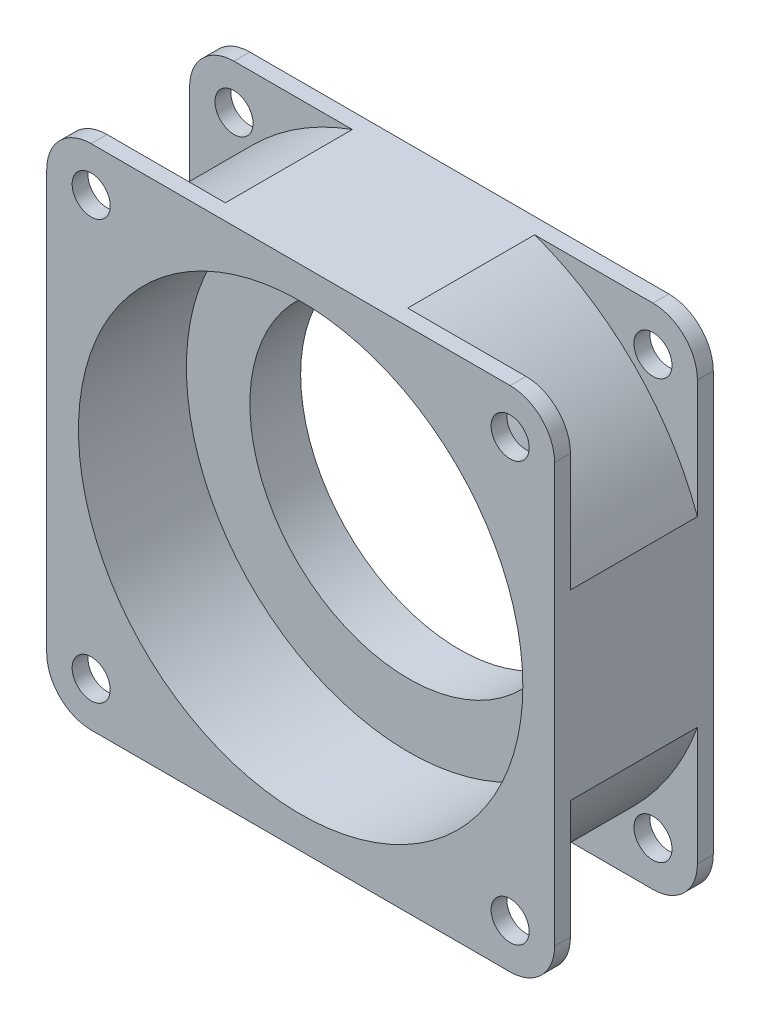
ISO-10303-21;
HEADER;
FILE_DESCRIPTION(('STEP AP214'),'2;1');
FILE_NAME('part.step','',(''),(''),'','','');
FILE_SCHEMA(('AUTOMOTIVE_DESIGN { 1 0 10303 214 1 1 1 1 }'));
ENDSEC;
DATA;
#1=APPLICATION_CONTEXT('core data for automotive mechanical design processes');
#2=APPLICATION_PROTOCOL_DEFINITION('international standard','automotive_design',2000,#1);
#3=PRODUCT_CONTEXT('',#1,'mechanical');
#4=PRODUCT('Part','Part','',(#3));
#5=PRODUCT_RELATED_PRODUCT_CATEGORY('part','',(#4));
#6=PRODUCT_DEFINITION_FORMATION('','',#4);
#7=PRODUCT_DEFINITION_CONTEXT('part definition',#1,'design');
#8=PRODUCT_DEFINITION('design','',#6,#7);
#9=PRODUCT_DEFINITION_SHAPE('','',#8);
#10=(LENGTH_UNIT() NAMED_UNIT(*) SI_UNIT(.MILLI.,.METRE.));
#11=(NAMED_UNIT(*) PLANE_ANGLE_UNIT() SI_UNIT($,.RADIAN.));
#12=(NAMED_UNIT(*) SI_UNIT($,.STERADIAN.) SOLID_ANGLE_UNIT());
#13=UNCERTAINTY_MEASURE_WITH_UNIT(LENGTH_MEASURE(1.E-05),#10,'distance_accuracy_value','');
#14=(GEOMETRIC_REPRESENTATION_CONTEXT(3) GLOBAL_UNCERTAINTY_ASSIGNED_CONTEXT((#13)) GLOBAL_UNIT_ASSIGNED_CONTEXT((#10,
#11,#12)) REPRESENTATION_CONTEXT('',''));
#15=CARTESIAN_POINT('',(0.,0.,0.));
#16=DIRECTION('',(0.,0.,1.));
#17=DIRECTION('',(1.,0.,0.));
#18=AXIS2_PLACEMENT_3D('',#15,#16,#17);
#19=CARTESIAN_POINT('',(0.,0.,-132.5));
#20=DIRECTION('',(0.,0.,1.));
#21=DIRECTION('',(1.,0.,0.));
#22=AXIS2_PLACEMENT_3D('',#19,#20,#21);
#23=CYLINDRICAL_SURFACE('',#22,25.);
#24=CARTESIAN_POINT('',(0.,0.,-25.));
#25=DIRECTION('',(0.,0.,-1.));
#26=DIRECTION('',(-1.,0.,0.));
#27=AXIS2_PLACEMENT_3D('',#24,#25,#26);
#28=CIRCLE('',#27,25.);
#29=CARTESIAN_POINT('',(-25.,0.,-25.));
#30=VERTEX_POINT('',#29);
#31=EDGE_CURVE('E363',#30,#30,#28,.T.);
#32=ORIENTED_EDGE('',*,*,#31,.T.);
#33=EDGE_LOOP('',(#32));
#34=FACE_BOUND('',#33,.T.);
#35=CARTESIAN_POINT('',(0.,0.,-17.));
#36=DIRECTION('',(0.,0.,1.));
#37=DIRECTION('',(1.,0.,0.));
#38=AXIS2_PLACEMENT_3D('',#35,#36,#37);
#39=CIRCLE('',#38,25.);
#40=CARTESIAN_POINT('',(25.,0.,-17.));
#41=VERTEX_POINT('',#40);
#42=EDGE_CURVE('E43',#41,#41,#39,.F.);
#43=ORIENTED_EDGE('',*,*,#42,.F.);
#44=EDGE_LOOP('',(#43));
#45=FACE_BOUND('',#44,.T.);
#46=ADVANCED_FACE('F39',(#34,#45),#23,.F.);
#47=CARTESIAN_POINT('',(33.,33.,-2.5));
#48=DIRECTION('',(0.,0.,-1.));
#49=DIRECTION('',(-1.,0.,0.));
#50=AXIS2_PLACEMENT_3D('',#47,#48,#49);
#51=PLANE('',#50);
#52=CARTESIAN_POINT('',(-33.,33.,-2.5));
#53=DIRECTION('',(0.,0.,-1.));
#54=DIRECTION('',(-1.,0.,0.));
#55=AXIS2_PLACEMENT_3D('',#52,#53,#54);
#56=CIRCLE('',#55,3.);
#57=CARTESIAN_POINT('',(-36.,33.,-2.5));
#58=VERTEX_POINT('',#57);
#59=EDGE_CURVE('E359',#58,#58,#56,.T.);
#60=ORIENTED_EDGE('',*,*,#59,.F.);
#61=EDGE_LOOP('',(#60));
#62=FACE_BOUND('',#61,.T.);
#63=CARTESIAN_POINT('',(0.,0.,-2.5));
#64=DIRECTION('',(0.,0.,-1.));
#65=DIRECTION('',(-1.,0.,0.));
#66=AXIS2_PLACEMENT_3D('',#63,#64,#65);
#67=CIRCLE('',#66,42.5);
#68=CARTESIAN_POINT('',(-40.,14.3614066163451,-2.5));
#69=VERTEX_POINT('',#68);
#70=CARTESIAN_POINT('',(-14.3614066163451,40.,-2.5));
#71=VERTEX_POINT('',#70);
#72=EDGE_CURVE('E229',#69,#71,#67,.T.);
#73=ORIENTED_EDGE('',*,*,#72,.F.);
#74=DIRECTION('',(0.,-1.,0.));
#75=VECTOR('',#74,1.);
#76=CARTESIAN_POINT('',(-40.,-33.,-2.5));
#77=LINE('',#76,#75);
#78=CARTESIAN_POINT('',(-40.,33.,-2.5));
#79=VERTEX_POINT('',#78);
#80=EDGE_CURVE('E287',#79,#69,#77,.T.);
#81=ORIENTED_EDGE('',*,*,#80,.F.);
#82=CARTESIAN_POINT('',(-33.,33.,-2.5));
#83=DIRECTION('',(0.,0.,1.));
#84=DIRECTION('',(-1.,0.,0.));
#85=AXIS2_PLACEMENT_3D('',#82,#83,#84);
#86=CIRCLE('',#85,7.);
#87=CARTESIAN_POINT('',(-32.9999999999999,40.,-2.5));
#88=VERTEX_POINT('',#87);
#89=EDGE_CURVE('E289',#88,#79,#86,.T.);
#90=ORIENTED_EDGE('',*,*,#89,.F.);
#91=DIRECTION('',(-1.,0.,0.));
#92=VECTOR('',#91,1.);
#93=CARTESIAN_POINT('',(-32.9999999999999,40.,-2.5));
#94=LINE('',#93,#92);
#95=EDGE_CURVE('E57',#71,#88,#94,.T.);
#96=ORIENTED_EDGE('',*,*,#95,.F.);
#97=EDGE_LOOP('',(#73,#81,#90,#96));
#98=FACE_BOUND('',#97,.T.);
#99=ADVANCED_FACE('F477',(#62,#98),#51,.T.);
#100=CARTESIAN_POINT('',(-33.,-33.,-2.5));
#101=DIRECTION('',(0.,0.,-1.));
#102=DIRECTION('',(-1.,0.,0.));
#103=AXIS2_PLACEMENT_3D('',#100,#101,#102);
#104=CIRCLE('',#103,3.);
#105=CARTESIAN_POINT('',(-36.,-33.,-2.5));
#106=VERTEX_POINT('',#105);
#107=EDGE_CURVE('E352',#106,#106,#104,.T.);
#108=ORIENTED_EDGE('',*,*,#107,.F.);
#109=EDGE_LOOP('',(#108));
#110=FACE_BOUND('',#109,.T.);
#111=CARTESIAN_POINT('',(0.,0.,-2.5));
#112=DIRECTION('',(0.,0.,-1.));
#113=DIRECTION('',(-1.,0.,0.));
#114=AXIS2_PLACEMENT_3D('',#111,#112,#113);
#115=CIRCLE('',#114,42.5);
#116=CARTESIAN_POINT('',(-14.3614066163451,-40.,-2.5));
#117=VERTEX_POINT('',#116);
#118=CARTESIAN_POINT('',(-40.,-14.3614066163451,-2.5));
#119=VERTEX_POINT('',#118);
#120=EDGE_CURVE('E242',#117,#119,#115,.T.);
#121=ORIENTED_EDGE('',*,*,#120,.F.);
#122=DIRECTION('',(1.,0.,0.));
#123=VECTOR('',#122,1.);
#124=CARTESIAN_POINT('',(-32.9999999999999,-40.,-2.5));
#125=LINE('',#124,#123);
#126=CARTESIAN_POINT('',(-32.9999999999999,-40.,-2.5));
#127=VERTEX_POINT('',#126);
#128=EDGE_CURVE('E300',#127,#117,#125,.T.);
#129=ORIENTED_EDGE('',*,*,#128,.F.);
#130=CARTESIAN_POINT('',(-33.,-33.,-2.5));
#131=DIRECTION('',(0.,0.,1.));
#132=DIRECTION('',(-1.,0.,0.));
#133=AXIS2_PLACEMENT_3D('',#130,#131,#132);
#134=CIRCLE('',#133,7.);
#135=CARTESIAN_POINT('',(-40.,-33.,-2.5));
#136=VERTEX_POINT('',#135);
#137=EDGE_CURVE('E291',#136,#127,#134,.T.);
#138=ORIENTED_EDGE('',*,*,#137,.F.);
#139=EDGE_CURVE('E288',#119,#136,#77,.T.);
#140=ORIENTED_EDGE('',*,*,#139,.F.);
#141=EDGE_LOOP('',(#121,#129,#138,#140));
#142=FACE_BOUND('',#141,.T.);
#143=ADVANCED_FACE('F472',(#110,#142),#51,.T.);
#144=CARTESIAN_POINT('',(33.,-33.,-2.5));
#145=DIRECTION('',(0.,0.,-1.));
#146=DIRECTION('',(-1.,0.,0.));
#147=AXIS2_PLACEMENT_3D('',#144,#145,#146);
#148=CIRCLE('',#147,3.);
#149=CARTESIAN_POINT('',(30.,-33.,-2.5));
#150=VERTEX_POINT('',#149);
#151=EDGE_CURVE('E405',#150,#150,#148,.T.);
#152=ORIENTED_EDGE('',*,*,#151,.F.);
#153=EDGE_LOOP('',(#152));
#154=FACE_BOUND('',#153,.T.);
#155=CARTESIAN_POINT('',(0.,0.,-2.5));
#156=DIRECTION('',(0.,0.,-1.));
#157=DIRECTION('',(-1.,0.,0.));
#158=AXIS2_PLACEMENT_3D('',#155,#156,#157);
#159=CIRCLE('',#158,42.5);
#160=CARTESIAN_POINT('',(40.,-14.3614066163451,-2.5));
#161=VERTEX_POINT('',#160);
#162=CARTESIAN_POINT('',(14.3614066163451,-40.,-2.5));
#163=VERTEX_POINT('',#162);
#164=EDGE_CURVE('E252',#161,#163,#159,.T.);
#165=ORIENTED_EDGE('',*,*,#164,.F.);
#166=DIRECTION('',(0.,1.,0.));
#167=VECTOR('',#166,1.);
#168=CARTESIAN_POINT('',(40.,-33.,-2.5));
#169=LINE('',#168,#167);
#170=CARTESIAN_POINT('',(40.,-33.,-2.5));
#171=VERTEX_POINT('',#170);
#172=EDGE_CURVE('E303',#171,#161,#169,.T.);
#173=ORIENTED_EDGE('',*,*,#172,.F.);
#174=CARTESIAN_POINT('',(33.,-33.,-2.5));
#175=DIRECTION('',(0.,0.,1.));
#176=DIRECTION('',(-1.,0.,0.));
#177=AXIS2_PLACEMENT_3D('',#174,#175,#176);
#178=CIRCLE('',#177,7.);
#179=CARTESIAN_POINT('',(33.,-40.,-2.5));
#180=VERTEX_POINT('',#179);
#181=EDGE_CURVE('E296',#180,#171,#178,.T.);
#182=ORIENTED_EDGE('',*,*,#181,.F.);
#183=EDGE_CURVE('E297',#163,#180,#125,.T.);
#184=ORIENTED_EDGE('',*,*,#183,.F.);
#185=EDGE_LOOP('',(#165,#173,#182,#184));
#186=FACE_BOUND('',#185,.T.);
#187=ADVANCED_FACE('F692',(#154,#186),#51,.T.);
#188=CARTESIAN_POINT('',(33.,33.,-2.5));
#189=DIRECTION('',(0.,0.,1.));
#190=DIRECTION('',(1.,0.,0.));
#191=AXIS2_PLACEMENT_3D('',#188,#189,#190);
#192=CYLINDRICAL_SURFACE('',#191,7.);
#193=CARTESIAN_POINT('',(33.,33.,0.));
#194=DIRECTION('',(0.,0.,1.));
#195=DIRECTION('',(-1.,0.,0.));
#196=AXIS2_PLACEMENT_3D('',#193,#194,#195);
#197=CIRCLE('',#196,7.);
#198=CARTESIAN_POINT('',(40.,33.,0.));
#199=VERTEX_POINT('',#198);
#200=CARTESIAN_POINT('',(33.,40.,0.));
#201=VERTEX_POINT('',#200);
#202=EDGE_CURVE('E276',#199,#201,#197,.T.);
#203=ORIENTED_EDGE('',*,*,#202,.F.);
#204=DIRECTION('',(0.,0.,1.));
#205=VECTOR('',#204,1.);
#206=CARTESIAN_POINT('',(40.,33.,-2.5));
#207=LINE('',#206,#205);
#208=CARTESIAN_POINT('',(40.,33.,-2.5));
#209=VERTEX_POINT('',#208);
#210=EDGE_CURVE('E11',#209,#199,#207,.T.);
#211=ORIENTED_EDGE('',*,*,#210,.F.);
#212=CARTESIAN_POINT('',(33.,33.,-2.5));
#213=DIRECTION('',(0.,0.,1.));
#214=DIRECTION('',(-1.,0.,0.));
#215=AXIS2_PLACEMENT_3D('',#212,#213,#214);
#216=CIRCLE('',#215,7.);
#217=CARTESIAN_POINT('',(33.,40.,-2.5));
#218=VERTEX_POINT('',#217);
#219=EDGE_CURVE('E278',#209,#218,#216,.T.);
#220=ORIENTED_EDGE('',*,*,#219,.T.);
#221=DIRECTION('',(0.,0.,1.));
#222=VECTOR('',#221,1.);
#223=CARTESIAN_POINT('',(33.,40.,-2.5));
#224=LINE('',#223,#222);
#225=EDGE_CURVE('E307',#218,#201,#224,.T.);
#226=ORIENTED_EDGE('',*,*,#225,.T.);
#227=EDGE_LOOP('',(#203,#211,#220,#226));
#228=FACE_BOUND('',#227,.T.);
#229=ADVANCED_FACE('F41',(#228),#192,.T.);
#230=CARTESIAN_POINT('',(40.,-33.,-2.5));
#231=DIRECTION('',(1.,0.,0.));
#232=DIRECTION('',(0.,0.,-1.));
#233=AXIS2_PLACEMENT_3D('',#230,#231,#232);
#234=PLANE('',#233);
#235=DIRECTION('',(0.,1.,0.));
#236=VECTOR('',#235,1.);
#237=CARTESIAN_POINT('',(40.,-33.,0.));
#238=LINE('',#237,#236);
#239=CARTESIAN_POINT('',(40.,-33.,0.));
#240=VERTEX_POINT('',#239);
#241=EDGE_CURVE('E283',#240,#199,#238,.T.);
#242=ORIENTED_EDGE('',*,*,#241,.F.);
#243=DIRECTION('',(0.,0.,1.));
#244=VECTOR('',#243,1.);
#245=CARTESIAN_POINT('',(40.,-33.,-2.5));
#246=LINE('',#245,#244);
#247=EDGE_CURVE('E48',#171,#240,#246,.T.);
#248=ORIENTED_EDGE('',*,*,#247,.F.);
#249=ORIENTED_EDGE('',*,*,#172,.T.);
#250=DIRECTION('',(0.,0.,1.));
#251=VECTOR('',#250,1.);
#252=CARTESIAN_POINT('',(40.,-14.3614066163451,-22.5));
#253=LINE('',#252,#251);
#254=CARTESIAN_POINT('',(40.,-14.3614066163451,-22.5));
#255=VERTEX_POINT('',#254);
#256=EDGE_CURVE('E268',#255,#161,#253,.T.);
#257=ORIENTED_EDGE('',*,*,#256,.F.);
#258=DIRECTION('',(0.,-1.,0.));
#259=VECTOR('',#258,1.);
#260=CARTESIAN_POINT('',(40.,-33.,-22.5));
#261=LINE('',#260,#259);
#262=CARTESIAN_POINT('',(40.,-33.,-22.5));
#263=VERTEX_POINT('',#262);
#264=EDGE_CURVE('E432',#255,#263,#261,.T.);
#265=ORIENTED_EDGE('',*,*,#264,.T.);
#266=DIRECTION('',(0.,0.,1.));
#267=VECTOR('',#266,1.);
#268=CARTESIAN_POINT('',(40.,-33.,-25.));
#269=LINE('',#268,#267);
#270=CARTESIAN_POINT('',(40.,-33.,-25.));
#271=VERTEX_POINT('',#270);
#272=EDGE_CURVE('E412',#271,#263,#269,.T.);
#273=ORIENTED_EDGE('',*,*,#272,.F.);
#274=DIRECTION('',(0.,-1.,0.));
#275=VECTOR('',#274,1.);
#276=CARTESIAN_POINT('',(40.,-33.,-25.));
#277=LINE('',#276,#275);
#278=CARTESIAN_POINT('',(40.,32.9999999999999,-25.));
#279=VERTEX_POINT('',#278);
#280=EDGE_CURVE('E219',#279,#271,#277,.T.);
#281=ORIENTED_EDGE('',*,*,#280,.F.);
#282=DIRECTION('',(0.,0.,1.));
#283=VECTOR('',#282,1.);
#284=CARTESIAN_POINT('',(40.,32.9999999999999,-25.));
#285=LINE('',#284,#283);
#286=CARTESIAN_POINT('',(40.,32.9999999999999,-22.5));
#287=VERTEX_POINT('',#286);
#288=EDGE_CURVE('E437',#279,#287,#285,.T.);
#289=ORIENTED_EDGE('',*,*,#288,.T.);
#290=CARTESIAN_POINT('',(40.,14.3614066163451,-22.5));
#291=VERTEX_POINT('',#290);
#292=EDGE_CURVE('E221',#287,#291,#261,.T.);
#293=ORIENTED_EDGE('',*,*,#292,.T.);
#294=DIRECTION('',(0.,0.,1.));
#295=VECTOR('',#294,1.);
#296=CARTESIAN_POINT('',(40.,14.3614066163451,-22.5));
#297=LINE('',#296,#295);
#298=CARTESIAN_POINT('',(40.,14.3614066163451,-2.5));
#299=VERTEX_POINT('',#298);
#300=EDGE_CURVE('E271',#291,#299,#297,.T.);
#301=ORIENTED_EDGE('',*,*,#300,.T.);
#302=EDGE_CURVE('E305',#299,#209,#169,.T.);
#303=ORIENTED_EDGE('',*,*,#302,.T.);
#304=ORIENTED_EDGE('',*,*,#210,.T.);
#305=EDGE_LOOP('',(#242,#248,#249,#257,#265,#273,#281,#289,#293,#301,#303,#304));
#306=FACE_BOUND('',#305,.T.);
#307=ADVANCED_FACE('F639',(#306),#234,.T.);
#308=CARTESIAN_POINT('',(33.,-33.,-2.5));
#309=DIRECTION('',(0.,0.,1.));
#310=DIRECTION('',(1.,0.,0.));
#311=AXIS2_PLACEMENT_3D('',#308,#309,#310);
#312=CYLINDRICAL_SURFACE('',#311,7.);
#313=CARTESIAN_POINT('',(33.,-33.,0.));
#314=DIRECTION('',(0.,0.,1.));
#315=DIRECTION('',(-1.,0.,0.));
#316=AXIS2_PLACEMENT_3D('',#313,#314,#315);
#317=CIRCLE('',#316,7.);
#318=CARTESIAN_POINT('',(33.,-40.,0.));
#319=VERTEX_POINT('',#318);
#320=EDGE_CURVE('E324',#319,#240,#317,.T.);
#321=ORIENTED_EDGE('',*,*,#320,.F.);
#322=DIRECTION('',(0.,0.,1.));
#323=VECTOR('',#322,1.);
#324=CARTESIAN_POINT('',(33.,-40.,-2.5));
#325=LINE('',#324,#323);
#326=EDGE_CURVE('E332',#180,#319,#325,.T.);
#327=ORIENTED_EDGE('',*,*,#326,.F.);
#328=ORIENTED_EDGE('',*,*,#181,.T.);
#329=ORIENTED_EDGE('',*,*,#247,.T.);
#330=EDGE_LOOP('',(#321,#327,#328,#329));
#331=FACE_BOUND('',#330,.T.);
#332=ADVANCED_FACE('F631',(#331),#312,.T.);
#333=CARTESIAN_POINT('',(-32.9999999999999,-40.,-2.5));
#334=DIRECTION('',(0.,-1.,0.));
#335=DIRECTION('',(0.,0.,-1.));
#336=AXIS2_PLACEMENT_3D('',#333,#334,#335);
#337=PLANE('',#336);
#338=DIRECTION('',(1.,0.,0.));
#339=VECTOR('',#338,1.);
#340=CARTESIAN_POINT('',(-32.9999999999999,-40.,0.));
#341=LINE('',#340,#339);
#342=CARTESIAN_POINT('',(-32.9999999999999,-40.,0.));
#343=VERTEX_POINT('',#342);
#344=EDGE_CURVE('E325',#343,#319,#341,.T.);
#345=ORIENTED_EDGE('',*,*,#344,.F.);
#346=DIRECTION('',(0.,0.,1.));
#347=VECTOR('',#346,1.);
#348=CARTESIAN_POINT('',(-32.9999999999999,-40.,-2.5));
#349=LINE('',#348,#347);
#350=EDGE_CURVE('E334',#127,#343,#349,.T.);
#351=ORIENTED_EDGE('',*,*,#350,.F.);
#352=ORIENTED_EDGE('',*,*,#128,.T.);
#353=DIRECTION('',(0.,0.,1.));
#354=VECTOR('',#353,1.);
#355=CARTESIAN_POINT('',(-14.3614066163451,-40.,-22.5));
#356=LINE('',#355,#354);
#357=CARTESIAN_POINT('',(-14.3614066163451,-40.,-22.5));
#358=VERTEX_POINT('',#357);
#359=EDGE_CURVE('E265',#358,#117,#356,.T.);
#360=ORIENTED_EDGE('',*,*,#359,.F.);
#361=DIRECTION('',(-1.,0.,0.));
#362=VECTOR('',#361,1.);
#363=CARTESIAN_POINT('',(-33.,-40.,-22.5));
#364=LINE('',#363,#362);
#365=CARTESIAN_POINT('',(-33.,-40.,-22.5));
#366=VERTEX_POINT('',#365);
#367=EDGE_CURVE('E417',#358,#366,#364,.T.);
#368=ORIENTED_EDGE('',*,*,#367,.T.);
#369=DIRECTION('',(0.,0.,1.));
#370=VECTOR('',#369,1.);
#371=CARTESIAN_POINT('',(-33.,-40.,-25.));
#372=LINE('',#371,#370);
#373=CARTESIAN_POINT('',(-33.,-40.,-25.));
#374=VERTEX_POINT('',#373);
#375=EDGE_CURVE('E211',#374,#366,#372,.T.);
#376=ORIENTED_EDGE('',*,*,#375,.F.);
#377=DIRECTION('',(-1.,0.,0.));
#378=VECTOR('',#377,1.);
#379=CARTESIAN_POINT('',(-33.,-40.,-25.));
#380=LINE('',#379,#378);
#381=CARTESIAN_POINT('',(32.9999999999999,-40.,-25.));
#382=VERTEX_POINT('',#381);
#383=EDGE_CURVE('E205',#382,#374,#380,.T.);
#384=ORIENTED_EDGE('',*,*,#383,.F.);
#385=DIRECTION('',(0.,0.,1.));
#386=VECTOR('',#385,1.);
#387=CARTESIAN_POINT('',(32.9999999999999,-40.,-25.));
#388=LINE('',#387,#386);
#389=CARTESIAN_POINT('',(32.9999999999999,-40.,-22.5));
#390=VERTEX_POINT('',#389);
#391=EDGE_CURVE('E208',#382,#390,#388,.T.);
#392=ORIENTED_EDGE('',*,*,#391,.T.);
#393=CARTESIAN_POINT('',(14.3614066163451,-40.,-22.5));
#394=VERTEX_POINT('',#393);
#395=EDGE_CURVE('E416',#390,#394,#364,.T.);
#396=ORIENTED_EDGE('',*,*,#395,.T.);
#397=DIRECTION('',(0.,0.,1.));
#398=VECTOR('',#397,1.);
#399=CARTESIAN_POINT('',(14.3614066163451,-40.,-22.5));
#400=LINE('',#399,#398);
#401=EDGE_CURVE('E264',#394,#163,#400,.T.);
#402=ORIENTED_EDGE('',*,*,#401,.T.);
#403=ORIENTED_EDGE('',*,*,#183,.T.);
#404=ORIENTED_EDGE('',*,*,#326,.T.);
#405=EDGE_LOOP('',(#345,#351,#352,#360,#368,#376,#384,#392,#396,#402,#403,#404));
#406=FACE_BOUND('',#405,.T.);
#407=ADVANCED_FACE('F202',(#406),#337,.T.);
#408=CARTESIAN_POINT('',(-33.,-33.,-2.5));
#409=DIRECTION('',(0.,0.,1.));
#410=DIRECTION('',(1.,0.,0.));
#411=AXIS2_PLACEMENT_3D('',#408,#409,#410);
#412=CYLINDRICAL_SURFACE('',#411,7.);
#413=CARTESIAN_POINT('',(-33.,-33.,0.));
#414=DIRECTION('',(0.,0.,1.));
#415=DIRECTION('',(-1.,0.,0.));
#416=AXIS2_PLACEMENT_3D('',#413,#414,#415);
#417=CIRCLE('',#416,7.);
#418=CARTESIAN_POINT('',(-40.,-33.,0.));
#419=VERTEX_POINT('',#418);
#420=EDGE_CURVE('E317',#419,#343,#417,.T.);
#421=ORIENTED_EDGE('',*,*,#420,.F.);
#422=DIRECTION('',(0.,0.,1.));
#423=VECTOR('',#422,1.);
#424=CARTESIAN_POINT('',(-40.,-33.,-2.5));
#425=LINE('',#424,#423);
#426=EDGE_CURVE('E333',#136,#419,#425,.T.);
#427=ORIENTED_EDGE('',*,*,#426,.F.);
#428=ORIENTED_EDGE('',*,*,#137,.T.);
#429=ORIENTED_EDGE('',*,*,#350,.T.);
#430=EDGE_LOOP('',(#421,#427,#428,#429));
#431=FACE_BOUND('',#430,.T.);
#432=ADVANCED_FACE('F467',(#431),#412,.T.);
#433=CARTESIAN_POINT('',(-40.,-33.,-2.5));
#434=DIRECTION('',(-1.,0.,0.));
#435=DIRECTION('',(0.,0.,1.));
#436=AXIS2_PLACEMENT_3D('',#433,#434,#435);
#437=PLANE('',#436);
#438=DIRECTION('',(0.,-1.,0.));
#439=VECTOR('',#438,1.);
#440=CARTESIAN_POINT('',(-40.,-33.,0.));
#441=LINE('',#440,#439);
#442=CARTESIAN_POINT('',(-40.,33.,0.));
#443=VERTEX_POINT('',#442);
#444=EDGE_CURVE('E316',#443,#419,#441,.T.);
#445=ORIENTED_EDGE('',*,*,#444,.F.);
#446=DIRECTION('',(0.,0.,1.));
#447=VECTOR('',#446,1.);
#448=CARTESIAN_POINT('',(-40.,33.,-2.5));
#449=LINE('',#448,#447);
#450=EDGE_CURVE('E340',#79,#443,#449,.T.);
#451=ORIENTED_EDGE('',*,*,#450,.F.);
#452=ORIENTED_EDGE('',*,*,#80,.T.);
#453=DIRECTION('',(0.,0.,1.));
#454=VECTOR('',#453,1.);
#455=CARTESIAN_POINT('',(-40.,14.3614066163451,-22.5));
#456=LINE('',#455,#454);
#457=CARTESIAN_POINT('',(-40.,14.3614066163451,-22.5));
#458=VERTEX_POINT('',#457);
#459=EDGE_CURVE('E248',#458,#69,#456,.T.);
#460=ORIENTED_EDGE('',*,*,#459,.F.);
#461=DIRECTION('',(0.,1.,0.));
#462=VECTOR('',#461,1.);
#463=CARTESIAN_POINT('',(-40.,-33.,-22.5));
#464=LINE('',#463,#462);
#465=CARTESIAN_POINT('',(-40.,33.,-22.5));
#466=VERTEX_POINT('',#465);
#467=EDGE_CURVE('E425',#458,#466,#464,.T.);
#468=ORIENTED_EDGE('',*,*,#467,.T.);
#469=DIRECTION('',(0.,0.,1.));
#470=VECTOR('',#469,1.);
#471=CARTESIAN_POINT('',(-40.,33.,-25.));
#472=LINE('',#471,#470);
#473=CARTESIAN_POINT('',(-40.,33.,-25.));
#474=VERTEX_POINT('',#473);
#475=EDGE_CURVE('E450',#474,#466,#472,.T.);
#476=ORIENTED_EDGE('',*,*,#475,.F.);
#477=DIRECTION('',(0.,1.,0.));
#478=VECTOR('',#477,1.);
#479=CARTESIAN_POINT('',(-40.,-33.,-25.));
#480=LINE('',#479,#478);
#481=CARTESIAN_POINT('',(-40.,-33.,-25.));
#482=VERTEX_POINT('',#481);
#483=EDGE_CURVE('E407',#482,#474,#480,.T.);
#484=ORIENTED_EDGE('',*,*,#483,.F.);
#485=DIRECTION('',(0.,0.,1.));
#486=VECTOR('',#485,1.);
#487=CARTESIAN_POINT('',(-40.,-33.,-25.));
#488=LINE('',#487,#486);
#489=CARTESIAN_POINT('',(-40.,-33.,-22.5));
#490=VERTEX_POINT('',#489);
#491=EDGE_CURVE('E235',#482,#490,#488,.T.);
#492=ORIENTED_EDGE('',*,*,#491,.T.);
#493=CARTESIAN_POINT('',(-40.,-14.3614066163451,-22.5));
#494=VERTEX_POINT('',#493);
#495=EDGE_CURVE('E421',#490,#494,#464,.T.);
#496=ORIENTED_EDGE('',*,*,#495,.T.);
#497=DIRECTION('',(0.,0.,1.));
#498=VECTOR('',#497,1.);
#499=CARTESIAN_POINT('',(-40.,-14.3614066163451,-22.5));
#500=LINE('',#499,#498);
#501=EDGE_CURVE('E259',#494,#119,#500,.T.);
#502=ORIENTED_EDGE('',*,*,#501,.T.);
#503=ORIENTED_EDGE('',*,*,#139,.T.);
#504=ORIENTED_EDGE('',*,*,#426,.T.);
#505=EDGE_LOOP('',(#445,#451,#452,#460,#468,#476,#484,#492,#496,#502,#503,#504));
#506=FACE_BOUND('',#505,.T.);
#507=ADVANCED_FACE('F452',(#506),#437,.T.);
#508=CARTESIAN_POINT('',(-33.,33.,-2.5));
#509=DIRECTION('',(0.,0.,1.));
#510=DIRECTION('',(1.,0.,0.));
#511=AXIS2_PLACEMENT_3D('',#508,#509,#510);
#512=CYLINDRICAL_SURFACE('',#511,7.);
#513=CARTESIAN_POINT('',(-33.,33.,0.));
#514=DIRECTION('',(0.,0.,1.));
#515=DIRECTION('',(-1.,0.,0.));
#516=AXIS2_PLACEMENT_3D('',#513,#514,#515);
#517=CIRCLE('',#516,7.);
#518=CARTESIAN_POINT('',(-32.9999999999999,40.,0.));
#519=VERTEX_POINT('',#518);
#520=EDGE_CURVE('E311',#519,#443,#517,.T.);
#521=ORIENTED_EDGE('',*,*,#520,.F.);
#522=DIRECTION('',(0.,0.,1.));
#523=VECTOR('',#522,1.);
#524=CARTESIAN_POINT('',(-32.9999999999999,40.,-2.5));
#525=LINE('',#524,#523);
#526=EDGE_CURVE('E339',#88,#519,#525,.T.);
#527=ORIENTED_EDGE('',*,*,#526,.F.);
#528=ORIENTED_EDGE('',*,*,#89,.T.);
#529=ORIENTED_EDGE('',*,*,#450,.T.);
#530=EDGE_LOOP('',(#521,#527,#528,#529));
#531=FACE_BOUND('',#530,.T.);
#532=ADVANCED_FACE('F485',(#531),#512,.T.);
#533=CARTESIAN_POINT('',(-32.9999999999999,40.,-2.5));
#534=DIRECTION('',(0.,1.,0.));
#535=DIRECTION('',(0.,0.,1.));
#536=AXIS2_PLACEMENT_3D('',#533,#534,#535);
#537=PLANE('',#536);
#538=DIRECTION('',(-1.,0.,0.));
#539=VECTOR('',#538,1.);
#540=CARTESIAN_POINT('',(-32.9999999999999,40.,0.));
#541=LINE('',#540,#539);
#542=EDGE_CURVE('E309',#201,#519,#541,.T.);
#543=ORIENTED_EDGE('',*,*,#542,.F.);
#544=ORIENTED_EDGE('',*,*,#225,.F.);
#545=CARTESIAN_POINT('',(14.3614066163451,40.,-2.5));
#546=VERTEX_POINT('',#545);
#547=EDGE_CURVE('E284',#218,#546,#94,.T.);
#548=ORIENTED_EDGE('',*,*,#547,.T.);
#549=DIRECTION('',(0.,0.,1.));
#550=VECTOR('',#549,1.);
#551=CARTESIAN_POINT('',(14.3614066163451,40.,-22.5));
#552=LINE('',#551,#550);
#553=CARTESIAN_POINT('',(14.3614066163451,40.,-22.5));
#554=VERTEX_POINT('',#553);
#555=EDGE_CURVE('E273',#554,#546,#552,.T.);
#556=ORIENTED_EDGE('',*,*,#555,.F.);
#557=DIRECTION('',(1.,0.,0.));
#558=VECTOR('',#557,1.);
#559=CARTESIAN_POINT('',(-33.,40.,-22.5));
#560=LINE('',#559,#558);
#561=CARTESIAN_POINT('',(32.9999999999999,40.,-22.5));
#562=VERTEX_POINT('',#561);
#563=EDGE_CURVE('E428',#554,#562,#560,.T.);
#564=ORIENTED_EDGE('',*,*,#563,.T.);
#565=DIRECTION('',(0.,0.,1.));
#566=VECTOR('',#565,1.);
#567=CARTESIAN_POINT('',(32.9999999999999,40.,-25.));
#568=LINE('',#567,#566);
#569=CARTESIAN_POINT('',(32.9999999999999,40.,-25.));
#570=VERTEX_POINT('',#569);
#571=EDGE_CURVE('E442',#570,#562,#568,.T.);
#572=ORIENTED_EDGE('',*,*,#571,.F.);
#573=DIRECTION('',(1.,0.,0.));
#574=VECTOR('',#573,1.);
#575=CARTESIAN_POINT('',(-33.,40.,-25.));
#576=LINE('',#575,#574);
#577=CARTESIAN_POINT('',(-33.,40.,-25.));
#578=VERTEX_POINT('',#577);
#579=EDGE_CURVE('E406',#578,#570,#576,.T.);
#580=ORIENTED_EDGE('',*,*,#579,.F.);
#581=DIRECTION('',(0.,0.,1.));
#582=VECTOR('',#581,1.);
#583=CARTESIAN_POINT('',(-33.,40.,-25.));
#584=LINE('',#583,#582);
#585=CARTESIAN_POINT('',(-33.,40.,-22.5));
#586=VERTEX_POINT('',#585);
#587=EDGE_CURVE('E441',#578,#586,#584,.T.);
#588=ORIENTED_EDGE('',*,*,#587,.T.);
#589=CARTESIAN_POINT('',(-14.3614066163451,40.,-22.5));
#590=VERTEX_POINT('',#589);
#591=EDGE_CURVE('E427',#586,#590,#560,.T.);
#592=ORIENTED_EDGE('',*,*,#591,.T.);
#593=DIRECTION('',(0.,0.,1.));
#594=VECTOR('',#593,1.);
#595=CARTESIAN_POINT('',(-14.3614066163451,40.,-22.5));
#596=LINE('',#595,#594);
#597=EDGE_CURVE('E280',#590,#71,#596,.T.);
#598=ORIENTED_EDGE('',*,*,#597,.T.);
#599=ORIENTED_EDGE('',*,*,#95,.T.);
#600=ORIENTED_EDGE('',*,*,#526,.T.);
#601=EDGE_LOOP('',(#543,#544,#548,#556,#564,#572,#580,#588,#592,#598,#599,#600));
#602=FACE_BOUND('',#601,.T.);
#603=ADVANCED_FACE('F484',(#602),#537,.T.);
#604=CARTESIAN_POINT('',(33.,33.,-2.5));
#605=DIRECTION('',(0.,0.,-1.));
#606=DIRECTION('',(-1.,0.,0.));
#607=AXIS2_PLACEMENT_3D('',#604,#605,#606);
#608=CIRCLE('',#607,3.);
#609=CARTESIAN_POINT('',(30.,33.,-2.5));
#610=VERTEX_POINT('',#609);
#611=EDGE_CURVE('E357',#610,#610,#608,.T.);
#612=ORIENTED_EDGE('',*,*,#611,.F.);
#613=EDGE_LOOP('',(#612));
#614=FACE_BOUND('',#613,.T.);
#615=CARTESIAN_POINT('',(0.,0.,-2.5));
#616=DIRECTION('',(0.,0.,-1.));
#617=DIRECTION('',(-1.,0.,0.));
#618=AXIS2_PLACEMENT_3D('',#615,#616,#617);
#619=CIRCLE('',#618,42.5);
#620=EDGE_CURVE('E64',#546,#299,#619,.T.);
#621=ORIENTED_EDGE('',*,*,#620,.F.);
#622=ORIENTED_EDGE('',*,*,#547,.F.);
#623=ORIENTED_EDGE('',*,*,#219,.F.);
#624=ORIENTED_EDGE('',*,*,#302,.F.);
#625=EDGE_LOOP('',(#621,#622,#623,#624));
#626=FACE_BOUND('',#625,.T.);
#627=ADVANCED_FACE('F522',(#614,#626),#51,.T.);
#628=CARTESIAN_POINT('',(33.,33.,0.));
#629=DIRECTION('',(0.,0.,-1.));
#630=DIRECTION('',(-1.,0.,0.));
#631=AXIS2_PLACEMENT_3D('',#628,#629,#630);
#632=PLANE('',#631);
#633=CARTESIAN_POINT('',(0.,0.,0.));
#634=DIRECTION('',(0.,0.,1.));
#635=DIRECTION('',(1.,0.,0.));
#636=AXIS2_PLACEMENT_3D('',#633,#634,#635);
#637=CIRCLE('',#636,35.);
#638=CARTESIAN_POINT('',(35.,0.,0.));
#639=VERTEX_POINT('',#638);
#640=EDGE_CURVE('E372',#639,#639,#637,.T.);
#641=ORIENTED_EDGE('',*,*,#640,.F.);
#642=EDGE_LOOP('',(#641));
#643=FACE_BOUND('',#642,.T.);
#644=CARTESIAN_POINT('',(-33.,-33.,0.));
#645=DIRECTION('',(0.,0.,1.));
#646=DIRECTION('',(1.,0.,0.));
#647=AXIS2_PLACEMENT_3D('',#644,#645,#646);
#648=CIRCLE('',#647,3.);
#649=CARTESIAN_POINT('',(-30.,-33.,0.));
#650=VERTEX_POINT('',#649);
#651=EDGE_CURVE('E361',#650,#650,#648,.T.);
#652=ORIENTED_EDGE('',*,*,#651,.F.);
#653=EDGE_LOOP('',(#652));
#654=FACE_BOUND('',#653,.T.);
#655=CARTESIAN_POINT('',(33.,-33.,0.));
#656=DIRECTION('',(0.,0.,1.));
#657=DIRECTION('',(1.,0.,0.));
#658=AXIS2_PLACEMENT_3D('',#655,#656,#657);
#659=CIRCLE('',#658,3.);
#660=CARTESIAN_POINT('',(36.,-33.,0.));
#661=VERTEX_POINT('',#660);
#662=EDGE_CURVE('E370',#661,#661,#659,.T.);
#663=ORIENTED_EDGE('',*,*,#662,.F.);
#664=EDGE_LOOP('',(#663));
#665=FACE_BOUND('',#664,.T.);
#666=CARTESIAN_POINT('',(33.,33.,0.));
#667=DIRECTION('',(0.,0.,1.));
#668=DIRECTION('',(1.,0.,0.));
#669=AXIS2_PLACEMENT_3D('',#666,#667,#668);
#670=CIRCLE('',#669,3.);
#671=CARTESIAN_POINT('',(36.,33.,0.));
#672=VERTEX_POINT('',#671);
#673=EDGE_CURVE('E381',#672,#672,#670,.T.);
#674=ORIENTED_EDGE('',*,*,#673,.F.);
#675=EDGE_LOOP('',(#674));
#676=FACE_BOUND('',#675,.T.);
#677=CARTESIAN_POINT('',(-33.,33.,0.));
#678=DIRECTION('',(0.,0.,1.));
#679=DIRECTION('',(1.,0.,0.));
#680=AXIS2_PLACEMENT_3D('',#677,#678,#679);
#681=CIRCLE('',#680,3.);
#682=CARTESIAN_POINT('',(-30.,33.,0.));
#683=VERTEX_POINT('',#682);
#684=EDGE_CURVE('E347',#683,#683,#681,.T.);
#685=ORIENTED_EDGE('',*,*,#684,.F.);
#686=EDGE_LOOP('',(#685));
#687=FACE_BOUND('',#686,.T.);
#688=ORIENTED_EDGE('',*,*,#202,.T.);
#689=ORIENTED_EDGE('',*,*,#542,.T.);
#690=ORIENTED_EDGE('',*,*,#520,.T.);
#691=ORIENTED_EDGE('',*,*,#444,.T.);
#692=ORIENTED_EDGE('',*,*,#420,.T.);
#693=ORIENTED_EDGE('',*,*,#344,.T.);
#694=ORIENTED_EDGE('',*,*,#320,.T.);
#695=ORIENTED_EDGE('',*,*,#241,.T.);
#696=EDGE_LOOP('',(#688,#689,#690,#691,#692,#693,#694,#695));
#697=FACE_BOUND('',#696,.T.);
#698=ADVANCED_FACE('F478',(#643,#654,#665,#676,#687,#697),#632,.F.);
#699=CARTESIAN_POINT('',(0.,0.,-22.5));
#700=DIRECTION('',(0.,0.,1.));
#701=DIRECTION('',(1.,0.,0.));
#702=AXIS2_PLACEMENT_3D('',#699,#700,#701);
#703=CYLINDRICAL_SURFACE('',#702,42.5);
#704=ORIENTED_EDGE('',*,*,#72,.T.);
#705=ORIENTED_EDGE('',*,*,#597,.F.);
#706=CARTESIAN_POINT('',(0.,0.,-22.5));
#707=DIRECTION('',(0.,0.,-1.));
#708=DIRECTION('',(-1.,0.,0.));
#709=AXIS2_PLACEMENT_3D('',#706,#707,#708);
#710=CIRCLE('',#709,42.5);
#711=EDGE_CURVE('E240',#458,#590,#710,.T.);
#712=ORIENTED_EDGE('',*,*,#711,.F.);
#713=ORIENTED_EDGE('',*,*,#459,.T.);
#714=EDGE_LOOP('',(#704,#705,#712,#713));
#715=FACE_BOUND('',#714,.T.);
#716=ADVANCED_FACE('F487',(#715),#703,.T.);
#717=CARTESIAN_POINT('',(0.,0.,-22.5));
#718=DIRECTION('',(0.,0.,1.));
#719=DIRECTION('',(1.,0.,0.));
#720=AXIS2_PLACEMENT_3D('',#717,#718,#719);
#721=CYLINDRICAL_SURFACE('',#720,42.5);
#722=ORIENTED_EDGE('',*,*,#620,.T.);
#723=ORIENTED_EDGE('',*,*,#300,.F.);
#724=CARTESIAN_POINT('',(0.,0.,-22.5));
#725=DIRECTION('',(0.,0.,-1.));
#726=DIRECTION('',(-1.,0.,0.));
#727=AXIS2_PLACEMENT_3D('',#724,#725,#726);
#728=CIRCLE('',#727,42.5);
#729=EDGE_CURVE('E238',#554,#291,#728,.T.);
#730=ORIENTED_EDGE('',*,*,#729,.F.);
#731=ORIENTED_EDGE('',*,*,#555,.T.);
#732=EDGE_LOOP('',(#722,#723,#730,#731));
#733=FACE_BOUND('',#732,.T.);
#734=ADVANCED_FACE('F664',(#733),#721,.T.);
#735=CARTESIAN_POINT('',(0.,0.,-22.5));
#736=DIRECTION('',(0.,0.,1.));
#737=DIRECTION('',(1.,0.,0.));
#738=AXIS2_PLACEMENT_3D('',#735,#736,#737);
#739=CYLINDRICAL_SURFACE('',#738,42.5);
#740=ORIENTED_EDGE('',*,*,#164,.T.);
#741=ORIENTED_EDGE('',*,*,#401,.F.);
#742=CARTESIAN_POINT('',(0.,0.,-22.5));
#743=DIRECTION('',(0.,0.,-1.));
#744=DIRECTION('',(-1.,0.,0.));
#745=AXIS2_PLACEMENT_3D('',#742,#743,#744);
#746=CIRCLE('',#745,42.5);
#747=EDGE_CURVE('E244',#255,#394,#746,.T.);
#748=ORIENTED_EDGE('',*,*,#747,.F.);
#749=ORIENTED_EDGE('',*,*,#256,.T.);
#750=EDGE_LOOP('',(#740,#741,#748,#749));
#751=FACE_BOUND('',#750,.T.);
#752=ADVANCED_FACE('F508',(#751),#739,.T.);
#753=CARTESIAN_POINT('',(0.,0.,-22.5));
#754=DIRECTION('',(0.,0.,1.));
#755=DIRECTION('',(1.,0.,0.));
#756=AXIS2_PLACEMENT_3D('',#753,#754,#755);
#757=CYLINDRICAL_SURFACE('',#756,42.5);
#758=ORIENTED_EDGE('',*,*,#120,.T.);
#759=ORIENTED_EDGE('',*,*,#501,.F.);
#760=CARTESIAN_POINT('',(0.,0.,-22.5));
#761=DIRECTION('',(0.,0.,-1.));
#762=DIRECTION('',(-1.,0.,0.));
#763=AXIS2_PLACEMENT_3D('',#760,#761,#762);
#764=CIRCLE('',#763,42.5);
#765=EDGE_CURVE('E246',#358,#494,#764,.T.);
#766=ORIENTED_EDGE('',*,*,#765,.F.);
#767=ORIENTED_EDGE('',*,*,#359,.T.);
#768=EDGE_LOOP('',(#758,#759,#766,#767));
#769=FACE_BOUND('',#768,.T.);
#770=ADVANCED_FACE('F464',(#769),#757,.T.);
#771=CARTESIAN_POINT('',(33.,-33.,-22.5));
#772=DIRECTION('',(0.,0.,-1.));
#773=DIRECTION('',(-1.,0.,0.));
#774=AXIS2_PLACEMENT_3D('',#771,#772,#773);
#775=PLANE('',#774);
#776=CARTESIAN_POINT('',(-33.,33.,-22.5));
#777=DIRECTION('',(0.,0.,-1.));
#778=DIRECTION('',(-1.,0.,0.));
#779=AXIS2_PLACEMENT_3D('',#776,#777,#778);
#780=CIRCLE('',#779,3.);
#781=CARTESIAN_POINT('',(-36.,33.,-22.5));
#782=VERTEX_POINT('',#781);
#783=EDGE_CURVE('E348',#782,#782,#780,.T.);
#784=ORIENTED_EDGE('',*,*,#783,.T.);
#785=EDGE_LOOP('',(#784));
#786=FACE_BOUND('',#785,.T.);
#787=ORIENTED_EDGE('',*,*,#467,.F.);
#788=ORIENTED_EDGE('',*,*,#711,.T.);
#789=ORIENTED_EDGE('',*,*,#591,.F.);
#790=CARTESIAN_POINT('',(-33.,33.,-22.5));
#791=DIRECTION('',(0.,0.,-1.));
#792=DIRECTION('',(-1.,0.,0.));
#793=AXIS2_PLACEMENT_3D('',#790,#791,#792);
#794=CIRCLE('',#793,7.);
#795=EDGE_CURVE('E426',#466,#586,#794,.T.);
#796=ORIENTED_EDGE('',*,*,#795,.F.);
#797=EDGE_LOOP('',(#787,#788,#789,#796));
#798=FACE_BOUND('',#797,.T.);
#799=ADVANCED_FACE('F500',(#786,#798),#775,.F.);
#800=CARTESIAN_POINT('',(33.,33.,-22.5));
#801=DIRECTION('',(0.,0.,-1.));
#802=DIRECTION('',(-1.,0.,0.));
#803=AXIS2_PLACEMENT_3D('',#800,#801,#802);
#804=CIRCLE('',#803,3.);
#805=CARTESIAN_POINT('',(30.,33.,-22.5));
#806=VERTEX_POINT('',#805);
#807=EDGE_CURVE('E351',#806,#806,#804,.T.);
#808=ORIENTED_EDGE('',*,*,#807,.T.);
#809=EDGE_LOOP('',(#808));
#810=FACE_BOUND('',#809,.T.);
#811=ORIENTED_EDGE('',*,*,#563,.F.);
#812=ORIENTED_EDGE('',*,*,#729,.T.);
#813=ORIENTED_EDGE('',*,*,#292,.F.);
#814=CARTESIAN_POINT('',(33.,33.,-22.5));
#815=DIRECTION('',(0.,0.,-1.));
#816=DIRECTION('',(1.,0.,0.));
#817=AXIS2_PLACEMENT_3D('',#814,#815,#816);
#818=CIRCLE('',#817,7.);
#819=EDGE_CURVE('E435',#562,#287,#818,.T.);
#820=ORIENTED_EDGE('',*,*,#819,.F.);
#821=EDGE_LOOP('',(#811,#812,#813,#820));
#822=FACE_BOUND('',#821,.T.);
#823=ADVANCED_FACE('F496',(#810,#822),#775,.F.);
#824=CARTESIAN_POINT('',(33.,-33.,-22.5));
#825=DIRECTION('',(0.,0.,-1.));
#826=DIRECTION('',(-1.,0.,0.));
#827=AXIS2_PLACEMENT_3D('',#824,#825,#826);
#828=CIRCLE('',#827,3.);
#829=CARTESIAN_POINT('',(30.,-33.,-22.5));
#830=VERTEX_POINT('',#829);
#831=EDGE_CURVE('E358',#830,#830,#828,.T.);
#832=ORIENTED_EDGE('',*,*,#831,.T.);
#833=EDGE_LOOP('',(#832));
#834=FACE_BOUND('',#833,.T.);
#835=ORIENTED_EDGE('',*,*,#264,.F.);
#836=ORIENTED_EDGE('',*,*,#747,.T.);
#837=ORIENTED_EDGE('',*,*,#395,.F.);
#838=CARTESIAN_POINT('',(33.,-33.,-22.5));
#839=DIRECTION('',(0.,0.,-1.));
#840=DIRECTION('',(-1.,0.,0.));
#841=AXIS2_PLACEMENT_3D('',#838,#839,#840);
#842=CIRCLE('',#841,7.);
#843=EDGE_CURVE('E228',#263,#390,#842,.T.);
#844=ORIENTED_EDGE('',*,*,#843,.F.);
#845=EDGE_LOOP('',(#835,#836,#837,#844));
#846=FACE_BOUND('',#845,.T.);
#847=ADVANCED_FACE('F509',(#834,#846),#775,.F.);
#848=CARTESIAN_POINT('',(33.,-33.,-25.));
#849=DIRECTION('',(0.,0.,1.));
#850=DIRECTION('',(1.,0.,0.));
#851=AXIS2_PLACEMENT_3D('',#848,#849,#850);
#852=CYLINDRICAL_SURFACE('',#851,7.);
#853=ORIENTED_EDGE('',*,*,#843,.T.);
#854=ORIENTED_EDGE('',*,*,#391,.F.);
#855=CARTESIAN_POINT('',(33.,-33.,-25.));
#856=DIRECTION('',(0.,0.,-1.));
#857=DIRECTION('',(-1.,0.,0.));
#858=AXIS2_PLACEMENT_3D('',#855,#856,#857);
#859=CIRCLE('',#858,7.);
#860=EDGE_CURVE('E214',#271,#382,#859,.T.);
#861=ORIENTED_EDGE('',*,*,#860,.F.);
#862=ORIENTED_EDGE('',*,*,#272,.T.);
#863=EDGE_LOOP('',(#853,#854,#861,#862));
#864=FACE_BOUND('',#863,.T.);
#865=ADVANCED_FACE('F227',(#864),#852,.T.);
#866=CARTESIAN_POINT('',(-33.,-33.,-25.));
#867=DIRECTION('',(0.,0.,1.));
#868=DIRECTION('',(1.,0.,0.));
#869=AXIS2_PLACEMENT_3D('',#866,#867,#868);
#870=CYLINDRICAL_SURFACE('',#869,7.);
#871=CARTESIAN_POINT('',(-33.,-33.,-22.5));
#872=DIRECTION('',(0.,0.,-1.));
#873=DIRECTION('',(1.,0.,0.));
#874=AXIS2_PLACEMENT_3D('',#871,#872,#873);
#875=CIRCLE('',#874,7.);
#876=EDGE_CURVE('E419',#366,#490,#875,.T.);
#877=ORIENTED_EDGE('',*,*,#876,.T.);
#878=ORIENTED_EDGE('',*,*,#491,.F.);
#879=CARTESIAN_POINT('',(-33.,-33.,-25.));
#880=DIRECTION('',(0.,0.,-1.));
#881=DIRECTION('',(1.,0.,0.));
#882=AXIS2_PLACEMENT_3D('',#879,#880,#881);
#883=CIRCLE('',#882,7.);
#884=EDGE_CURVE('E212',#374,#482,#883,.T.);
#885=ORIENTED_EDGE('',*,*,#884,.F.);
#886=ORIENTED_EDGE('',*,*,#375,.T.);
#887=EDGE_LOOP('',(#877,#878,#885,#886));
#888=FACE_BOUND('',#887,.T.);
#889=ADVANCED_FACE('F785',(#888),#870,.T.);
#890=CARTESIAN_POINT('',(-33.,33.,-25.));
#891=DIRECTION('',(0.,0.,1.));
#892=DIRECTION('',(1.,0.,0.));
#893=AXIS2_PLACEMENT_3D('',#890,#891,#892);
#894=CYLINDRICAL_SURFACE('',#893,7.);
#895=ORIENTED_EDGE('',*,*,#795,.T.);
#896=ORIENTED_EDGE('',*,*,#587,.F.);
#897=CARTESIAN_POINT('',(-33.,33.,-25.));
#898=DIRECTION('',(0.,0.,-1.));
#899=DIRECTION('',(-1.,0.,0.));
#900=AXIS2_PLACEMENT_3D('',#897,#898,#899);
#901=CIRCLE('',#900,7.);
#902=EDGE_CURVE('E408',#474,#578,#901,.T.);
#903=ORIENTED_EDGE('',*,*,#902,.F.);
#904=ORIENTED_EDGE('',*,*,#475,.T.);
#905=EDGE_LOOP('',(#895,#896,#903,#904));
#906=FACE_BOUND('',#905,.T.);
#907=ADVANCED_FACE('F494',(#906),#894,.T.);
#908=CARTESIAN_POINT('',(33.,33.,-25.));
#909=DIRECTION('',(0.,0.,1.));
#910=DIRECTION('',(1.,0.,0.));
#911=AXIS2_PLACEMENT_3D('',#908,#909,#910);
#912=CYLINDRICAL_SURFACE('',#911,7.);
#913=ORIENTED_EDGE('',*,*,#819,.T.);
#914=ORIENTED_EDGE('',*,*,#288,.F.);
#915=CARTESIAN_POINT('',(33.,33.,-25.));
#916=DIRECTION('',(0.,0.,-1.));
#917=DIRECTION('',(1.,0.,0.));
#918=AXIS2_PLACEMENT_3D('',#915,#916,#917);
#919=CIRCLE('',#918,7.);
#920=EDGE_CURVE('E411',#570,#279,#919,.T.);
#921=ORIENTED_EDGE('',*,*,#920,.F.);
#922=ORIENTED_EDGE('',*,*,#571,.T.);
#923=EDGE_LOOP('',(#913,#914,#921,#922));
#924=FACE_BOUND('',#923,.T.);
#925=ADVANCED_FACE('F549',(#924),#912,.T.);
#926=CARTESIAN_POINT('',(33.,-33.,-25.));
#927=DIRECTION('',(0.,0.,-1.));
#928=DIRECTION('',(-1.,0.,0.));
#929=AXIS2_PLACEMENT_3D('',#926,#927,#928);
#930=PLANE('',#929);
#931=ORIENTED_EDGE('',*,*,#31,.F.);
#932=EDGE_LOOP('',(#931));
#933=FACE_BOUND('',#932,.T.);
#934=CARTESIAN_POINT('',(-33.,-33.,-25.));
#935=DIRECTION('',(0.,0.,-1.));
#936=DIRECTION('',(-1.,0.,0.));
#937=AXIS2_PLACEMENT_3D('',#934,#935,#936);
#938=CIRCLE('',#937,3.);
#939=CARTESIAN_POINT('',(-36.,-33.,-25.));
#940=VERTEX_POINT('',#939);
#941=EDGE_CURVE('E342',#940,#940,#938,.T.);
#942=ORIENTED_EDGE('',*,*,#941,.F.);
#943=EDGE_LOOP('',(#942));
#944=FACE_BOUND('',#943,.T.);
#945=CARTESIAN_POINT('',(33.,-33.,-25.));
#946=DIRECTION('',(0.,0.,-1.));
#947=DIRECTION('',(-1.,0.,0.));
#948=AXIS2_PLACEMENT_3D('',#945,#946,#947);
#949=CIRCLE('',#948,3.);
#950=CARTESIAN_POINT('',(30.,-33.,-25.));
#951=VERTEX_POINT('',#950);
#952=EDGE_CURVE('E356',#951,#951,#949,.T.);
#953=ORIENTED_EDGE('',*,*,#952,.F.);
#954=EDGE_LOOP('',(#953));
#955=FACE_BOUND('',#954,.T.);
#956=CARTESIAN_POINT('',(33.,33.,-25.));
#957=DIRECTION('',(0.,0.,-1.));
#958=DIRECTION('',(-1.,0.,0.));
#959=AXIS2_PLACEMENT_3D('',#956,#957,#958);
#960=CIRCLE('',#959,3.);
#961=CARTESIAN_POINT('',(30.,33.,-25.));
#962=VERTEX_POINT('',#961);
#963=EDGE_CURVE('E355',#962,#962,#960,.T.);
#964=ORIENTED_EDGE('',*,*,#963,.F.);
#965=EDGE_LOOP('',(#964));
#966=FACE_BOUND('',#965,.T.);
#967=CARTESIAN_POINT('',(-33.,33.,-25.));
#968=DIRECTION('',(0.,0.,-1.));
#969=DIRECTION('',(-1.,0.,0.));
#970=AXIS2_PLACEMENT_3D('',#967,#968,#969);
#971=CIRCLE('',#970,3.);
#972=CARTESIAN_POINT('',(-36.,33.,-25.));
#973=VERTEX_POINT('',#972);
#974=EDGE_CURVE('E350',#973,#973,#971,.T.);
#975=ORIENTED_EDGE('',*,*,#974,.F.);
#976=EDGE_LOOP('',(#975));
#977=FACE_BOUND('',#976,.T.);
#978=ORIENTED_EDGE('',*,*,#860,.T.);
#979=ORIENTED_EDGE('',*,*,#383,.T.);
#980=ORIENTED_EDGE('',*,*,#884,.T.);
#981=ORIENTED_EDGE('',*,*,#483,.T.);
#982=ORIENTED_EDGE('',*,*,#902,.T.);
#983=ORIENTED_EDGE('',*,*,#579,.T.);
#984=ORIENTED_EDGE('',*,*,#920,.T.);
#985=ORIENTED_EDGE('',*,*,#280,.T.);
#986=EDGE_LOOP('',(#978,#979,#980,#981,#982,#983,#984,#985));
#987=FACE_BOUND('',#986,.T.);
#988=ADVANCED_FACE('F217',(#933,#944,#955,#966,#977,#987),#930,.T.);
#989=CARTESIAN_POINT('',(-33.,-33.,-22.5));
#990=DIRECTION('',(0.,0.,-1.));
#991=DIRECTION('',(-1.,0.,0.));
#992=AXIS2_PLACEMENT_3D('',#989,#990,#991);
#993=CIRCLE('',#992,3.);
#994=CARTESIAN_POINT('',(-36.,-33.,-22.5));
#995=VERTEX_POINT('',#994);
#996=EDGE_CURVE('E341',#995,#995,#993,.T.);
#997=ORIENTED_EDGE('',*,*,#996,.T.);
#998=EDGE_LOOP('',(#997));
#999=FACE_BOUND('',#998,.T.);
#1000=ORIENTED_EDGE('',*,*,#367,.F.);
#1001=ORIENTED_EDGE('',*,*,#765,.T.);
#1002=ORIENTED_EDGE('',*,*,#495,.F.);
#1003=ORIENTED_EDGE('',*,*,#876,.F.);
#1004=EDGE_LOOP('',(#1000,#1001,#1002,#1003));
#1005=FACE_BOUND('',#1004,.T.);
#1006=ADVANCED_FACE('F462',(#999,#1005),#775,.F.);
#1007=CARTESIAN_POINT('',(-33.,-33.,-92.5));
#1008=DIRECTION('',(0.,0.,1.));
#1009=DIRECTION('',(1.,0.,0.));
#1010=AXIS2_PLACEMENT_3D('',#1007,#1008,#1009);
#1011=CYLINDRICAL_SURFACE('',#1010,3.);
#1012=ORIENTED_EDGE('',*,*,#941,.T.);
#1013=EDGE_LOOP('',(#1012));
#1014=FACE_BOUND('',#1013,.T.);
#1015=ORIENTED_EDGE('',*,*,#996,.F.);
#1016=EDGE_LOOP('',(#1015));
#1017=FACE_BOUND('',#1016,.T.);
#1018=ADVANCED_FACE('F514',(#1014,#1017),#1011,.F.);
#1019=CARTESIAN_POINT('',(-33.,33.,-92.5));
#1020=DIRECTION('',(0.,0.,1.));
#1021=DIRECTION('',(1.,0.,0.));
#1022=AXIS2_PLACEMENT_3D('',#1019,#1020,#1021);
#1023=CYLINDRICAL_SURFACE('',#1022,3.);
#1024=ORIENTED_EDGE('',*,*,#974,.T.);
#1025=EDGE_LOOP('',(#1024));
#1026=FACE_BOUND('',#1025,.T.);
#1027=ORIENTED_EDGE('',*,*,#783,.F.);
#1028=EDGE_LOOP('',(#1027));
#1029=FACE_BOUND('',#1028,.T.);
#1030=ADVANCED_FACE('F548',(#1026,#1029),#1023,.F.);
#1031=CARTESIAN_POINT('',(33.,33.,-92.5));
#1032=DIRECTION('',(0.,0.,1.));
#1033=DIRECTION('',(1.,0.,0.));
#1034=AXIS2_PLACEMENT_3D('',#1031,#1032,#1033);
#1035=CYLINDRICAL_SURFACE('',#1034,3.);
#1036=ORIENTED_EDGE('',*,*,#963,.T.);
#1037=EDGE_LOOP('',(#1036));
#1038=FACE_BOUND('',#1037,.T.);
#1039=ORIENTED_EDGE('',*,*,#807,.F.);
#1040=EDGE_LOOP('',(#1039));
#1041=FACE_BOUND('',#1040,.T.);
#1042=ADVANCED_FACE('F540',(#1038,#1041),#1035,.F.);
#1043=CARTESIAN_POINT('',(33.,-33.,-92.5));
#1044=DIRECTION('',(0.,0.,1.));
#1045=DIRECTION('',(1.,0.,0.));
#1046=AXIS2_PLACEMENT_3D('',#1043,#1044,#1045);
#1047=CYLINDRICAL_SURFACE('',#1046,3.);
#1048=ORIENTED_EDGE('',*,*,#952,.T.);
#1049=EDGE_LOOP('',(#1048));
#1050=FACE_BOUND('',#1049,.T.);
#1051=ORIENTED_EDGE('',*,*,#831,.F.);
#1052=EDGE_LOOP('',(#1051));
#1053=FACE_BOUND('',#1052,.T.);
#1054=ADVANCED_FACE('F545',(#1050,#1053),#1047,.F.);
#1055=ORIENTED_EDGE('',*,*,#59,.T.);
#1056=EDGE_LOOP('',(#1055));
#1057=FACE_BOUND('',#1056,.T.);
#1058=ORIENTED_EDGE('',*,*,#684,.T.);
#1059=EDGE_LOOP('',(#1058));
#1060=FACE_BOUND('',#1059,.T.);
#1061=ADVANCED_FACE('F532',(#1057,#1060),#1023,.F.);
#1062=ORIENTED_EDGE('',*,*,#611,.T.);
#1063=EDGE_LOOP('',(#1062));
#1064=FACE_BOUND('',#1063,.T.);
#1065=ORIENTED_EDGE('',*,*,#673,.T.);
#1066=EDGE_LOOP('',(#1065));
#1067=FACE_BOUND('',#1066,.T.);
#1068=ADVANCED_FACE('F533',(#1064,#1067),#1035,.F.);
#1069=ORIENTED_EDGE('',*,*,#151,.T.);
#1070=EDGE_LOOP('',(#1069));
#1071=FACE_BOUND('',#1070,.T.);
#1072=ORIENTED_EDGE('',*,*,#662,.T.);
#1073=EDGE_LOOP('',(#1072));
#1074=FACE_BOUND('',#1073,.T.);
#1075=ADVANCED_FACE('F534',(#1071,#1074),#1047,.F.);
#1076=ORIENTED_EDGE('',*,*,#107,.T.);
#1077=EDGE_LOOP('',(#1076));
#1078=FACE_BOUND('',#1077,.T.);
#1079=ORIENTED_EDGE('',*,*,#651,.T.);
#1080=EDGE_LOOP('',(#1079));
#1081=FACE_BOUND('',#1080,.T.);
#1082=ADVANCED_FACE('F539',(#1078,#1081),#1011,.F.);
#1083=CARTESIAN_POINT('',(0.,0.,-17.));
#1084=DIRECTION('',(0.,0.,1.));
#1085=DIRECTION('',(1.,0.,0.));
#1086=AXIS2_PLACEMENT_3D('',#1083,#1084,#1085);
#1087=PLANE('',#1086);
#1088=CARTESIAN_POINT('',(0.,0.,-17.));
#1089=DIRECTION('',(0.,0.,1.));
#1090=DIRECTION('',(1.,0.,0.));
#1091=AXIS2_PLACEMENT_3D('',#1088,#1089,#1090);
#1092=CIRCLE('',#1091,35.);
#1093=CARTESIAN_POINT('',(35.,0.,-17.));
#1094=VERTEX_POINT('',#1093);
#1095=EDGE_CURVE('E367',#1094,#1094,#1092,.T.);
#1096=ORIENTED_EDGE('',*,*,#1095,.T.);
#1097=EDGE_LOOP('',(#1096));
#1098=FACE_BOUND('',#1097,.T.);
#1099=ORIENTED_EDGE('',*,*,#42,.T.);
#1100=EDGE_LOOP('',(#1099));
#1101=FACE_BOUND('',#1100,.T.);
#1102=ADVANCED_FACE('F544',(#1098,#1101),#1087,.T.);
#1103=CARTESIAN_POINT('',(0.,0.,-17.));
#1104=DIRECTION('',(0.,0.,1.));
#1105=DIRECTION('',(1.,0.,0.));
#1106=AXIS2_PLACEMENT_3D('',#1103,#1104,#1105);
#1107=CYLINDRICAL_SURFACE('',#1106,35.);
#1108=ORIENTED_EDGE('',*,*,#1095,.F.);
#1109=EDGE_LOOP('',(#1108));
#1110=FACE_BOUND('',#1109,.T.);
#1111=ORIENTED_EDGE('',*,*,#640,.T.);
#1112=EDGE_LOOP('',(#1111));
#1113=FACE_BOUND('',#1112,.T.);
#1114=ADVANCED_FACE('F530',(#1110,#1113),#1107,.F.);
#1115=CLOSED_SHELL('',(#46,#99,#143,#187,#229,#307,#332,#407,#432,#507,#532,#603,#627,#698,#716,
#734,#752,#770,#799,#823,#847,#865,#889,#907,#925,#988,#1006,#1018,#1030,#1042,#1054,#1061,
#1068,#1075,#1082,#1102,#1114));
#1116=MANIFOLD_SOLID_BREP('B2',#1115);
#1117=ADVANCED_BREP_SHAPE_REPRESENTATION('',(#18,#1116),#14);
#1118=SHAPE_DEFINITION_REPRESENTATION(#9,#1117);
ENDSEC;
END-ISO-10303-21;
